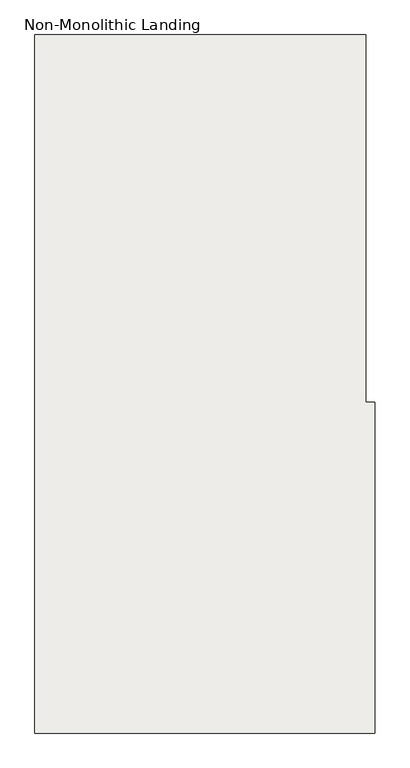
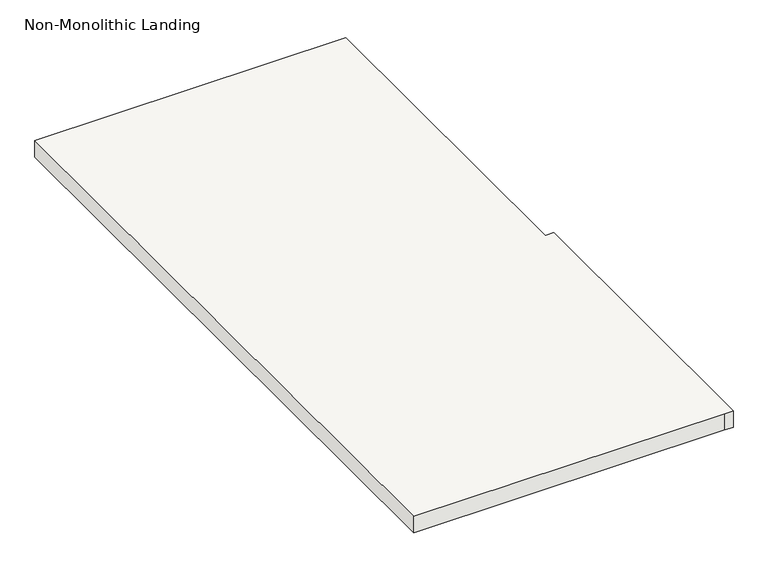
"""IFC4 building model written with IfcOpenShell, lengths in millimetres: slab geometry, Non-Monolithic Landing."""

from ifc_helpers import new_model, si_unit, origin, place, context, project, spatial, faceted_brep, source, transform, mapped, element, save


def non_monolithic_landing_6f2487d3(model_context):
    return source(origin(), model_context, "Body", "Brep", [
        faceted_brep([(-6392.3473712, -4870.057676, 4800.6), (-6392.3473712, -6800.457676, 4800.6), (-5477.9473712, -6800.457676, 4800.6), (-5452.5473712, -6800.457676, 4800.6), (-5452.5473712, -5886.057676, 4800.6), (-5477.9473712, -5886.057676, 4800.6), (-5477.9473712, -4870.057676, 4800.6), (-5503.3473712, -5784.457676, 4749.8), (-5477.9473712, -5784.457676, 4749.8), (-5477.9473712, -5886.057676, 4749.8), (-5452.5473712, -5886.057676, 4749.8), (-5452.5473712, -6800.457676, 4749.8), (-5477.9473712, -6800.457676, 4749.8), (-6392.3473712, -6800.457676, 4749.8), (-6392.3473712, -4870.057676, 4749.8), (-5503.3473712, -4870.057676, 4749.8), (-5477.9473712, -5784.457676, 4781.55), (-5477.9473712, -4870.057676, 4781.55), (-5503.3473712, -4870.057676, 4756.15), (-5503.3473712, -5784.457676, 4756.15)], [[[0, 1, 2, 3, 4, 5, 6]], [[7, 8, 9, 10, 11, 12, 13, 14, 15]], [[2, 1, 13, 12]], [[4, 3, 11, 10]], [[3, 2, 12, 11]], [[6, 5, 9, 8, 16, 17]], [[0, 6, 17, 18, 15, 14]], [[18, 17, 16, 19]], [[8, 7, 19, 16]], [[7, 15, 18, 19]], [[1, 0, 14, 13]], [[5, 4, 10, 9]]]),
    ])


if __name__ == "__main__":
    model = new_model("IFC4")
    model_context = context("Model", 3, world=origin())
    ifc_project = project(units=[si_unit("LENGTHUNIT", "METRE", prefix="MILLI")], contexts=[model_context])
    site = spatial("IfcSite", under=ifc_project)
    building = spatial("IfcBuilding", under=site)
    placement = place(None, origin())
    non_monolithic_landing_shape = non_monolithic_landing_6f2487d3(model_context)
    element("IfcSlab", 1, ObjectType="Non-Monolithic Landing", at=placement, inside=building, context=model_context, shape_type="MappedRepresentation", body=[
        mapped(non_monolithic_landing_shape, transform((0.0, 0.0, 0.0), x_axis=(1.0, 0.0, 0.0), y_axis=(0.0, 1.0, 0.0), z_axis=(0.0, 0.0, 1.0))),
    ])
    save(model, "model.ifc")
